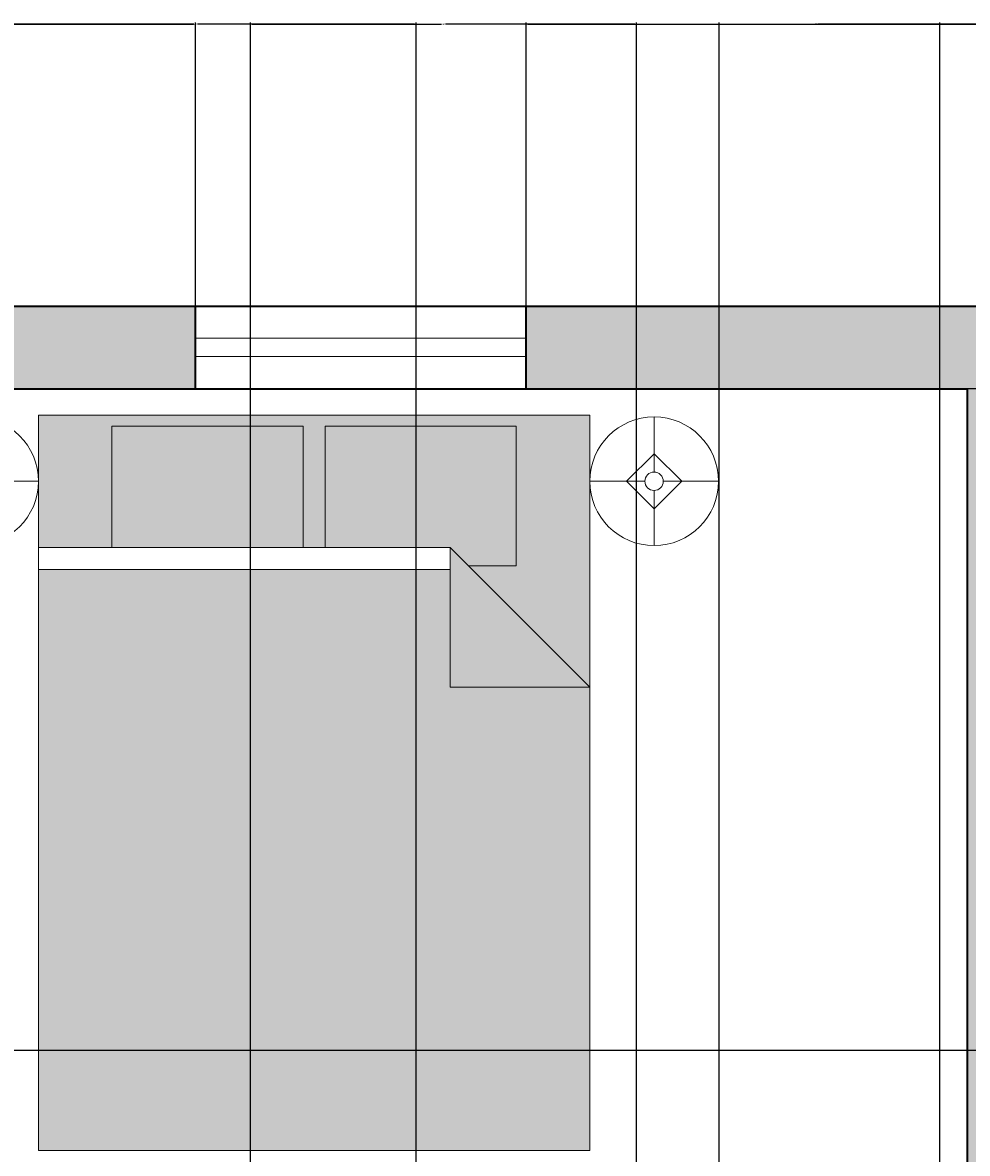
# Model space of a CAD drawing. Units: inches. Extents: x 1567 to 1964, y 1813 to 2447.
# Tile 15 of 28: x 1636 to 1738, y 2324 to 2447. Entities that reach past the tile are written whole.
import ezdxf

# ---------------------------------------------------------------- set-up
doc = ezdxf.new("R2010")
doc.units = ezdxf.units.IN
for name, color, linetype, lineweight in [('A-ANNO-DIMS', 2, 'Continuous', 18), ('A-FURN', 8, 'Continuous', 18), ('A-GLAZ', 4, 'Continuous', 18), ('A-WALL', 7, 'Continuous', 35)]:
    doc.layers.add(name, color=color, linetype=linetype, lineweight=lineweight)
doc.layers.add('A-FURN-PATT', color=252, linetype='Continuous', lineweight=13, true_color=0x939598)
doc.layers.add('A-WALL-PATT', color=251, linetype='Continuous', lineweight=13, true_color=0x636466)
doc.styles.get("Standard").update_dxf_attribs({"font": 'arial.ttf'})
doc.dimstyles.get("Standard").update_dxf_attribs({"dimtxt": 0.18, "dimasz": 0.18, "dimexe": 0.18, "dimexo": 0.0625, "dimgap": 0.09, "dimtad": 0, "dimtih": 1, "dimtoh": 1, "dimdec": 4, "dimzin": 0, "dimdsep": 46, "dimtxsty": 'Standard', "dimcen": 0.09, "dimadec": 0, "dimazin": 0, "dimtfac": 1, "dimtdec": 4, "dimtofl": 0, "dimtmove": 0, "dimatfit": 3, "dimfxl": 1, "dimtolj": 1, "dimtzin": 0, "dimarcsym": 0})

# ---------------------------------------------------------------- blocks, each defined once
blk = doc.blocks.new('Lamp - Table')
for p, q in [((0, 7), (0, 1)), ((0, 3), (-3, 0)), ((3, 0), (0, 3)), ((-1, 0), (-7, 0)), ((-3, 0), (0, -3)), ((0, -3), (3, 0)), ((1, 0), (7, 0)), ((0, -1), (0, -7))]:
    blk.add_line(p, q)
for radius in [7, 1]:
    blk.add_circle((0, 0), radius)
blk = doc.blocks.new('Bed - Queen')
for p, q in [((0, -80.00003), (0, 0)), ((0, 0), (59.99999, 0)), ((59.99999, 0), (59.99999, -80.00003)), ((7.99999, -1.2), (28.79998, -1.2)), ((7.99999, -14.4), (7.99999, -1.2)), ((28.79998, -1.2), (28.79998, -14.4)), ((31.19999, -1.2), (51.99999, -1.2)), ((31.19999, -14.4), (31.19999, -1.2)), ((51.99999, -1.2), (51.99999, -16.4)), ((0, -14.4), (44.8, -14.4)), ((59.99999, -29.6), (44.8, -14.4)), ((44.8, -14.4), (44.8, -29.6)), ((44.8, -16.8), (0, -16.8)), ((51.99999, -16.4), (46.79936, -16.4)), ((44.8, -29.6), (59.99999, -29.6)), ((59.99999, -80.00003), (0, -80.00003))]:
    blk.add_line(p, q)
blk = doc.blocks.new('WINDOW-36IN')
for p, q in [((0, 2), (36, 2)), ((0, 0), (36, 0))]:
    blk.add_line(p, q)
blk = doc.blocks.new('*D43')
at = {"layer": 'A-ANNO-DIMS', "color": 0, "lineweight": -2, "transparency": 16777216}
for p, q in [((1597.43, 2416.35), (1597.43, 2447.12)), ((1597.61, 2446.94), (1625.71, 2446.94)), ((1654.25, 2446.94), (1626.15, 2446.94)), ((1654.43, 2416.35), (1654.43, 2447.12))]:
    blk.add_line(p, q, dxfattribs=at)
at = {"layer": 'A-ANNO-DIMS', "color": 0, "transparency": 16777216}
for points in [[(1597.61, 2446.97), (1597.61, 2446.91), (1597.43, 2446.94)], [(1654.25, 2446.97), (1654.25, 2446.91), (1654.43, 2446.94)]]:
    blk.add_solid(points, dxfattribs=at)
at = {"layer": 'Defpoints', "color": 0, "transparency": 16777216}
for p in [(1654.43, 2446.94), (1597.43, 2416.29), (1654.43, 2416.29)]:
    blk.add_point(p, dxfattribs=at)
at = {"layer": 'A-ANNO-DIMS', "color": 0, "transparency": 16777216, "insert": (1625.93, 2446.94), "char_height": 0.18, "attachment_point": 5}
blk.add_mtext('\\A1;57', dxfattribs=at)
blk = doc.blocks.new('*D44')
at = {"layer": 'A-ANNO-DIMS', "color": 0, "lineweight": -2, "transparency": 16777216}
for p, q in [((1690.43, 2416.35), (1690.43, 2447.12)), ((1690.61, 2446.94), (1721.71, 2446.94)), ((1753.25, 2446.94), (1722.15, 2446.94)), ((1753.43, 2416.35), (1753.43, 2447.12))]:
    blk.add_line(p, q, dxfattribs=at)
at = {"layer": 'A-ANNO-DIMS', "color": 0, "transparency": 16777216}
for points in [[(1690.61, 2446.97), (1690.61, 2446.91), (1690.43, 2446.94)], [(1753.25, 2446.97), (1753.25, 2446.91), (1753.43, 2446.94)]]:
    blk.add_solid(points, dxfattribs=at)
at = {"layer": 'Defpoints', "color": 0, "transparency": 16777216}
for p in [(1753.43, 2446.94), (1690.43, 2416.29), (1753.43, 2416.29)]:
    blk.add_point(p, dxfattribs=at)
at = {"layer": 'A-ANNO-DIMS', "color": 0, "transparency": 16777216, "insert": (1721.93, 2446.94), "char_height": 0.18, "attachment_point": 5}
blk.add_mtext('\\A1;63', dxfattribs=at)
blk = doc.blocks.new('*D48')
at = {"layer": 'A-ANNO-DIMS', "color": 0, "lineweight": -2, "transparency": 16777216}
for p, q in [((1742.37, 2407.29), (1566.6, 2407.29)), ((1566.78, 2407.11), (1566.78, 2371.47)), ((1566.78, 2335.47), (1566.78, 2371.11)), ((1742.37, 2335.29), (1566.6, 2335.29))]:
    blk.add_line(p, q, dxfattribs=at)
at = {"layer": 'A-ANNO-DIMS', "color": 0, "transparency": 16777216}
for points in [[(1566.75, 2407.11), (1566.81, 2407.11), (1566.78, 2407.29)], [(1566.75, 2335.47), (1566.81, 2335.47), (1566.78, 2335.29)]]:
    blk.add_solid(points, dxfattribs=at)
at = {"layer": 'Defpoints', "color": 0, "transparency": 16777216}
for p in [(1742.43, 2407.29), (1566.78, 2335.29), (1742.43, 2335.29)]:
    blk.add_point(p, dxfattribs=at)
at = {"layer": 'A-ANNO-DIMS', "color": 0, "transparency": 16777216, "insert": (1566.78, 2371.29), "char_height": 0.18, "attachment_point": 5}
blk.add_mtext('\\A1;72', dxfattribs=at)
blk = doc.blocks.new('*D54')
at = {"layer": 'A-ANNO-DIMS', "color": 0, "lineweight": -2, "transparency": 16777216}
for p, q in [((1711.43, 1964.35), (1711.43, 2447.12)), ((1711.61, 2446.94), (1753.21, 2446.94)), ((1795.25, 2446.94), (1753.65, 2446.94)), ((1795.43, 1964.35), (1795.43, 2447.12))]:
    blk.add_line(p, q, dxfattribs=at)
at = {"layer": 'A-ANNO-DIMS', "color": 0, "transparency": 16777216}
for points in [[(1711.61, 2446.97), (1711.61, 2446.91), (1711.43, 2446.94)], [(1795.25, 2446.97), (1795.25, 2446.91), (1795.43, 2446.94)]]:
    blk.add_solid(points, dxfattribs=at)
at = {"layer": 'Defpoints', "color": 0, "transparency": 16777216}
for p in [(1795.43, 2446.94), (1711.43, 1964.29), (1795.43, 1964.29)]:
    blk.add_point(p, dxfattribs=at)
at = {"layer": 'A-ANNO-DIMS', "color": 0, "transparency": 16777216, "insert": (1753.43, 2446.94), "char_height": 0.18, "attachment_point": 5}
blk.add_mtext('\\A1;84', dxfattribs=at)
blk = doc.blocks.new('*D57')
at = {"layer": 'A-ANNO-DIMS', "color": 0, "lineweight": -2, "transparency": 16777216}
for p, q in [((1630.43, 2127.35), (1630.43, 2447.12)), ((1630.61, 2446.94), (1654.21, 2446.94)), ((1678.25, 2446.94), (1654.65, 2446.94)), ((1678.43, 2127.35), (1678.43, 2447.12))]:
    blk.add_line(p, q, dxfattribs=at)
at = {"layer": 'A-ANNO-DIMS', "color": 0, "transparency": 16777216}
for points in [[(1630.61, 2446.97), (1630.61, 2446.91), (1630.43, 2446.94)], [(1678.25, 2446.97), (1678.25, 2446.91), (1678.43, 2446.94)]]:
    blk.add_solid(points, dxfattribs=at)
at = {"layer": 'Defpoints', "color": 0, "transparency": 16777216}
for p in [(1678.43, 2446.94), (1630.43, 2127.29), (1678.43, 2127.29)]:
    blk.add_point(p, dxfattribs=at)
at = {"layer": 'A-ANNO-DIMS', "color": 0, "transparency": 16777216, "insert": (1654.43, 2446.94), "char_height": 0.18, "attachment_point": 5}
blk.add_mtext('\\A1;48', dxfattribs=at)
blk = doc.blocks.new('*D60')
at = {"layer": 'A-ANNO-DIMS', "color": 0, "lineweight": -2, "transparency": 16777216}
for p, q in [((1660.43, 2063.35), (1660.43, 2447.12)), ((1660.61, 2446.94), (1681.21, 2446.94)), ((1702.25, 2446.94), (1681.65, 2446.94)), ((1702.43, 2063.35), (1702.43, 2447.12))]:
    blk.add_line(p, q, dxfattribs=at)
at = {"layer": 'A-ANNO-DIMS', "color": 0, "transparency": 16777216}
for points in [[(1660.61, 2446.97), (1660.61, 2446.91), (1660.43, 2446.94)], [(1702.25, 2446.97), (1702.25, 2446.91), (1702.43, 2446.94)]]:
    blk.add_solid(points, dxfattribs=at)
at = {"layer": 'Defpoints', "color": 0, "transparency": 16777216}
for p in [(1660.43, 2446.94), (1660.43, 2063.29), (1702.43, 2063.29)]:
    blk.add_point(p, dxfattribs=at)
at = {"layer": 'A-ANNO-DIMS', "color": 0, "transparency": 16777216, "insert": (1681.43, 2446.94), "char_height": 0.18, "attachment_point": 5}
blk.add_mtext('\\A1;42', dxfattribs=at)
blk = doc.blocks.new('*D63')
at = {"layer": 'A-ANNO-DIMS', "color": 0, "lineweight": -2, "transparency": 16777216}
for p, q in [((1735.43, 1988.35), (1735.43, 2447.12)), ((1735.61, 2446.94), (1753.21, 2446.94)), ((1771.25, 2446.94), (1753.65, 2446.94)), ((1771.43, 1988.35), (1771.43, 2447.12))]:
    blk.add_line(p, q, dxfattribs=at)
at = {"layer": 'A-ANNO-DIMS', "color": 0, "transparency": 16777216}
for points in [[(1735.61, 2446.97), (1735.61, 2446.91), (1735.43, 2446.94)], [(1771.25, 2446.97), (1771.25, 2446.91), (1771.43, 2446.94)]]:
    blk.add_solid(points, dxfattribs=at)
at = {"layer": 'Defpoints', "color": 0, "transparency": 16777216}
for p in [(1771.43, 2446.94), (1735.43, 1988.29), (1771.43, 1988.29)]:
    blk.add_point(p, dxfattribs=at)
at = {"layer": 'A-ANNO-DIMS', "color": 0, "transparency": 16777216, "insert": (1753.43, 2446.94), "char_height": 0.18, "attachment_point": 5}
blk.add_mtext('\\A1;36', dxfattribs=at)
blk = doc.blocks.new('*D64')
at = {"layer": 'A-ANNO-DIMS', "color": 0, "lineweight": -2, "transparency": 16777216}
for p, q in [((1711.43, 2055.85), (1711.43, 2447.12)), ((1711.61, 2446.94), (1723.21, 2446.94)), ((1735.25, 2446.94), (1723.65, 2446.94)), ((1735.43, 2055.85), (1735.43, 2447.12))]:
    blk.add_line(p, q, dxfattribs=at)
at = {"layer": 'A-ANNO-DIMS', "color": 0, "transparency": 16777216}
for points in [[(1711.61, 2446.97), (1711.61, 2446.91), (1711.43, 2446.94)], [(1735.25, 2446.97), (1735.25, 2446.91), (1735.43, 2446.94)]]:
    blk.add_solid(points, dxfattribs=at)
at = {"layer": 'Defpoints', "color": 0, "transparency": 16777216}
for p in [(1735.43, 2446.94), (1711.43, 2055.79), (1735.43, 2055.79)]:
    blk.add_point(p, dxfattribs=at)
at = {"layer": 'A-ANNO-DIMS', "color": 0, "transparency": 16777216, "insert": (1723.43, 2446.94), "char_height": 0.18, "attachment_point": 5}
blk.add_mtext('\\A1;24', dxfattribs=at)

msp = doc.modelspace()

# ---------------------------------------------------------------- hatches: boundary and pattern name
at = {"layer": 'A-FURN-PATT'}
h = msp.add_hatch(color=256, dxfattribs=at)
h.dxf.hatch_style = 1
h.paths.add_polyline_path([(1621.2532, 2242.0229), (1643.7811, 2241.7239), (1643.8607, 2247.7234), (1617.863, 2248.0685, 0.19047621), (1616.7481, 2164.0759), (1642.7458, 2163.7308), (1642.8254, 2169.7302), (1620.2975, 2170.0293, -0.15194781)])
h.paths.add_polyline_path([(1673.5306, 2249.6607), (1653.8509, 2249.6607), (1653.8509, 2248.5031, 0.11764706), (1673.5306, 2248.5031)])
h.paths.add_polyline_path([(1706.0889, 2249.6607), (1686.4092, 2249.6607), (1686.4092, 2248.5031, 0.11764706), (1706.0889, 2248.5031)])
h.paths.add_polyline_path([(1782.4511, 2227.4197), (1766.4511, 2227.4197), (1766.2949, 2226.4197), (1782.6074, 2226.4197)])
h.paths.add_polyline_path([(1810.4511, 2227.4197), (1794.4511, 2227.4197), (1794.2949, 2226.4197), (1810.6074, 2226.4197)])
h.paths.add_polyline_path([(1743.9511, 2208.076), (1742.9511, 2207.9197), (1742.9511, 2191.9197), (1743.9511, 2191.7635)])
h.paths.add_polyline_path([(1782.6074, 2173.4197), (1766.2949, 2173.4197), (1766.4511, 2172.4197), (1782.4511, 2172.4197)])
h.paths.add_polyline_path([(1810.6074, 2173.4197), (1794.2949, 2173.4197), (1794.4511, 2172.4197), (1810.4511, 2172.4197)])
h.paths.add_polyline_path([(1861.053, 2006.5071), (1845.8531, 2006.5071), (1861.053, 1991.3071)])
h.paths.add_polyline_path([(1905.853, 1993.7071), (1861.053, 1993.7071), (1861.053, 1991.3071), (1905.853, 1991.3071)])
h.paths.add_polyline_path([(1919.7245, 2257.29, 0.50000012), (1918.7245, 2258.29), (1901.7245, 2258.29, 0.50000012), (1900.7245, 2257.29), (1900.7245, 2253.29, 0.50000012), (1901.7245, 2252.29), (1918.7245, 2252.29, 0.50000012), (1919.7245, 2253.29)])
h.paths.add_polyline_path([(1875.9094, 2391.0204), (1875.9094, 2375.8204), (1891.1093, 2375.8204)], flags=17)
h.paths.add_polyline_path([(1891.1093, 2405.4204), (1831.1094, 2405.4204), (1831.1094, 2391.0204), (1839.1093, 2391.0204), (1839.1093, 2404.2204), (1859.9093, 2404.2204), (1859.9093, 2391.0204), (1862.3093, 2391.0204), (1862.3093, 2404.2204), (1883.1093, 2404.2204), (1883.1093, 2389.0204), (1877.9094, 2389.0204), (1891.1093, 2375.8204)])
h.paths.add_polyline_path([(1682.1402, 2390.0316), (1682.1402, 2374.8316), (1697.3402, 2374.8316)], flags=17)
h.paths.add_polyline_path([(1697.3402, 2404.4316), (1637.3402, 2404.4316), (1637.3402, 2390.0316), (1645.3402, 2390.0316), (1645.3402, 2403.2316), (1666.1402, 2403.2316), (1666.1402, 2390.0316), (1668.5402, 2390.0316), (1668.5402, 2403.2316), (1689.3402, 2403.2316), (1689.3402, 2388.0316), (1684.1402, 2388.0316), (1697.3402, 2374.8316)])
h = msp.add_hatch(color=256, dxfattribs=at)
h.dxf.hatch_style = 1
h.paths.add_polyline_path([(1666.1402, 2403.2316), (1645.3402, 2403.2316), (1645.3402, 2390.0316), (1666.1402, 2390.0316)])
h.paths.add_polyline_path([(1689.3402, 2403.2316), (1668.5402, 2403.2316), (1668.5402, 2390.0316), (1682.1402, 2390.0316), (1684.1402, 2388.0316), (1689.3402, 2388.0316)])
h.paths.add_polyline_path([(1859.9093, 2404.2204), (1839.1093, 2404.2204), (1839.1093, 2391.0204), (1859.9093, 2391.0204)])
h.paths.add_polyline_path([(1883.1093, 2404.2204), (1862.3093, 2404.2204), (1862.3093, 2391.0204), (1875.9094, 2391.0204), (1877.9094, 2389.0204), (1883.1093, 2389.0204)])
h = msp.add_hatch(color=256, dxfattribs=at)
h.dxf.hatch_style = 1
h.paths.add_polyline_path([(1697.3402, 2374.8316), (1682.1402, 2374.8316), (1682.1402, 2387.6316), (1637.3402, 2387.6316), (1637.3402, 2324.4315), (1697.3402, 2324.4315)])
h.paths.add_polyline_path([(1891.1093, 2375.8204), (1875.9094, 2375.8204), (1875.9094, 2388.6204), (1831.1094, 2388.6204), (1831.1094, 2325.4204), (1891.1093, 2325.4204)])
h.paths.add_polyline_path([(1702.5611, 2206.8057), (1702.5611, 2210.8057), (1699.7395, 2209.9436), (1697.013, 2209.2403), (1694.3857, 2208.6763), (1691.8615, 2208.2326), (1689.4443, 2207.8896), (1687.1381, 2207.6282), (1684.9469, 2207.4289), (1682.8747, 2207.2725), (1680.9233, 2207.1425), (1679.0865, 2207.0339), (1677.3558, 2206.9445), (1675.7229, 2206.8719), (1674.1794, 2206.8141), (1672.7169, 2206.7688), (1671.327, 2206.7339), (1670.0014, 2206.707), (1668.7314, 2206.6866), (1667.5072, 2206.6732), (1666.3188, 2206.668), (1665.1561, 2206.6722), (1664.009, 2206.6869), (1662.8675, 2206.7133), (1661.7215, 2206.7525), (1660.5611, 2206.8057), (1660.5611, 2202.8057), (1661.9932, 2202.9556), (1663.3314, 2203.0744), (1664.5899, 2203.1671), (1665.7831, 2203.2385), (1666.9254, 2203.2935), (1668.0311, 2203.3368), (1669.1145, 2203.3734), (1670.1902, 2203.4081), (1671.2724, 2203.4451), (1672.3759, 2203.4866), (1673.5155, 2203.534), (1674.706, 2203.5887), (1675.9621, 2203.6523), (1677.2986, 2203.7262), (1678.7304, 2203.8118), (1680.2722, 2203.9108), (1681.947, 2204.0272), (1683.8108, 2204.1769), (1685.9279, 2204.3782), (1688.3626, 2204.6496), (1691.179, 2205.0096), (1694.4413, 2205.4767), (1698.214, 2206.0692)])
h.paths.add_polyline_path([(1702.5611, 2218.8057), (1701.9821, 2217.9383), (1701.3316, 2217.191), (1700.6091, 2216.5515), (1699.8141, 2216.0071), (1698.946, 2215.5454), (1698.0041, 2215.1536), (1696.9879, 2214.8194), (1695.8969, 2214.5301), (1694.7328, 2214.2753), (1693.5072, 2214.0522), (1692.2339, 2213.8602), (1690.9266, 2213.6989), (1689.5994, 2213.5675), (1688.266, 2213.4654), (1686.9402, 2213.392), (1685.636, 2213.3467), (1684.3619, 2213.3287), (1683.1053, 2213.3361), (1681.8482, 2213.3668), (1680.5727, 2213.4187), (1679.2608, 2213.4898), (1677.8948, 2213.5779), (1676.4565, 2213.6811), (1674.9282, 2213.7971), (1673.2982, 2213.9236), (1671.5804, 2214.0573), (1669.795, 2214.1945), (1667.9622, 2214.3316), (1666.1022, 2214.4649), (1664.2352, 2214.5908), (1662.3814, 2214.7056), (1660.5611, 2214.8057), (1660.5611, 2206.8057), (1661.7215, 2206.7525), (1662.8675, 2206.7133), (1664.009, 2206.6869), (1665.1561, 2206.6722), (1666.3188, 2206.668), (1667.5072, 2206.6732), (1668.7314, 2206.6866), (1670.0014, 2206.707), (1671.327, 2206.7339), (1672.7169, 2206.7688), (1674.1794, 2206.8141), (1675.7229, 2206.8719), (1677.3558, 2206.9445), (1679.0865, 2207.0339), (1680.9233, 2207.1425), (1682.8747, 2207.2725), (1684.9469, 2207.4289), (1687.1381, 2207.6282), (1689.4443, 2207.8896), (1691.8615, 2208.2326), (1694.3857, 2208.6763), (1697.013, 2209.2403), (1699.7395, 2209.9436), (1702.5611, 2210.8057)])
h.paths.add_polyline_path([(1700.6091, 2216.5515), (1701.3316, 2217.191), (1701.9821, 2217.9383), (1702.5611, 2218.8057), (1702.5611, 2222.8057), (1689.452, 2222.8057), (1689.0171, 2222.4556), (1688.4521, 2222.0354), (1687.7806, 2221.5662), (1687.0235, 2221.067), (1686.2019, 2220.5566), (1685.3367, 2220.0541), (1684.4491, 2219.5785), (1683.56, 2219.1486), (1682.6867, 2218.7795), (1681.8312, 2218.4692), (1680.9918, 2218.212), (1680.1667, 2218.0019), (1679.3541, 2217.833), (1678.5524, 2217.6995), (1677.7597, 2217.5954), (1676.9744, 2217.5149), (1676.1942, 2217.4531), (1675.4146, 2217.4093), (1674.6309, 2217.384), (1673.8381, 2217.3774), (1673.0313, 2217.39), (1672.2056, 2217.4221), (1671.3562, 2217.4741), (1670.4782, 2217.5463), (1669.5642, 2217.639), (1668.5968, 2217.7516), (1667.5562, 2217.8833), (1666.4226, 2218.0336), (1665.1761, 2218.2017), (1663.7969, 2218.3869), (1662.2651, 2218.5885), (1660.5611, 2218.8057), (1660.5611, 2214.8057), (1662.3814, 2214.7056), (1664.2352, 2214.5908), (1666.1022, 2214.4649), (1667.9622, 2214.3316), (1669.795, 2214.1945), (1671.5804, 2214.0573), (1673.2982, 2213.9236), (1674.9282, 2213.7971), (1676.4565, 2213.6811), (1677.8948, 2213.5779), (1679.2608, 2213.4898), (1680.5727, 2213.4187), (1681.8482, 2213.3668), (1683.1053, 2213.3361), (1684.3619, 2213.3287), (1685.636, 2213.3467), (1686.9402, 2213.392), (1688.266, 2213.4654), (1689.5994, 2213.5675), (1690.9266, 2213.6989), (1692.2339, 2213.8602), (1693.5072, 2214.0522), (1694.7328, 2214.2753), (1695.8969, 2214.5301), (1696.9879, 2214.8194), (1698.0041, 2215.1536), (1698.946, 2215.5454), (1699.8141, 2216.0071)])
h.paths.add_polyline_path([(1687.0235, 2221.067), (1687.7806, 2221.5662), (1688.4521, 2222.0354), (1689.0171, 2222.4556), (1689.452, 2222.8057), (1660.5611, 2222.8057), (1660.5611, 2218.8057), (1662.2651, 2218.5885), (1663.7969, 2218.3869), (1665.1761, 2218.2017), (1666.4226, 2218.0336), (1667.5562, 2217.8833), (1668.5968, 2217.7516), (1669.5642, 2217.639), (1670.4782, 2217.5463), (1671.3562, 2217.4741), (1672.2056, 2217.4221), (1673.0313, 2217.39), (1673.8381, 2217.3774), (1674.6309, 2217.384), (1675.4146, 2217.4093), (1676.1942, 2217.4531), (1676.9744, 2217.5149), (1677.7597, 2217.5954), (1678.5524, 2217.6995), (1679.3541, 2217.833), (1680.1667, 2218.0019), (1680.9918, 2218.212), (1681.8312, 2218.4692), (1682.6867, 2218.7795), (1683.56, 2219.1486), (1684.4491, 2219.5785), (1685.3367, 2220.0541), (1686.2019, 2220.5566)], flags=17)
h.paths.add_polyline_path([(1702.5611, 2198.8057), (1698.9289, 2199.2412), (1695.8472, 2199.5774), (1693.2166, 2199.8257), (1690.9377, 2199.9973), (1688.9111, 2200.1033), (1687.0375, 2200.155), (1685.2174, 2200.1637), (1683.3514, 2200.1406), (1681.3514, 2200.0941), (1679.1736, 2200.0225), (1676.7858, 2199.921), (1674.1554, 2199.7852), (1671.2502, 2199.6103), (1668.0377, 2199.3919), (1664.4854, 2199.1252), (1660.5611, 2198.8057), (1660.5611, 2194.8057), (1662.2697, 2194.9771), (1663.9673, 2195.0999), (1665.6339, 2195.1809), (1667.2495, 2195.227), (1668.7941, 2195.2449), (1670.2478, 2195.2414), (1671.5906, 2195.2233), (1672.8026, 2195.1974), (1673.8739, 2195.1689), (1674.8359, 2195.1364), (1675.7302, 2195.0967), (1676.5982, 2195.0469), (1677.4817, 2194.9838), (1678.422, 2194.9043), (1679.4609, 2194.8055), (1680.6397, 2194.6842), (1682.005, 2194.5341), (1683.6223, 2194.335), (1685.562, 2194.0637), (1687.8945, 2193.6967), (1690.6902, 2193.2108), (1694.0196, 2192.5826), (1697.9531, 2191.7887), (1702.5611, 2190.8057)])
h.paths.add_polyline_path([(1702.5611, 2206.8057), (1698.214, 2206.0692), (1694.4413, 2205.4767), (1691.179, 2205.0096), (1688.3626, 2204.6496), (1685.9279, 2204.3782), (1683.8108, 2204.1769), (1681.947, 2204.0272), (1680.2722, 2203.9108), (1678.7304, 2203.8118), (1677.2986, 2203.7262), (1675.9621, 2203.6523), (1674.706, 2203.5887), (1673.5155, 2203.534), (1672.3759, 2203.4866), (1671.2724, 2203.4451), (1670.1902, 2203.4081), (1669.1145, 2203.3734), (1668.0311, 2203.3368), (1666.9254, 2203.2935), (1665.7831, 2203.2385), (1664.5899, 2203.1671), (1663.3314, 2203.0744), (1661.9932, 2202.9556), (1660.5611, 2202.8057), (1660.5611, 2198.8057), (1664.4854, 2199.1252), (1668.0377, 2199.3919), (1671.2502, 2199.6103), (1674.1554, 2199.7852), (1676.7858, 2199.921), (1679.1736, 2200.0225), (1681.3514, 2200.0941), (1683.3514, 2200.1406), (1685.2174, 2200.1637), (1687.0375, 2200.155), (1688.9111, 2200.1033), (1690.9377, 2199.9973), (1693.2166, 2199.8257), (1695.8472, 2199.5774), (1698.9289, 2199.2412), (1702.5611, 2198.8057)])
h.paths.add_polyline_path([(1702.5611, 2190.8057), (1697.9531, 2191.7887), (1694.0196, 2192.5826), (1690.6902, 2193.2108), (1687.8945, 2193.6967), (1685.562, 2194.0637), (1683.6223, 2194.335), (1682.005, 2194.5341), (1680.6397, 2194.6842), (1679.4609, 2194.8055), (1678.422, 2194.9043), (1677.4817, 2194.9838), (1676.5982, 2195.0469), (1675.7302, 2195.0967), (1674.8359, 2195.1364), (1673.8739, 2195.1689), (1672.8026, 2195.1974), (1671.5906, 2195.2233), (1670.2478, 2195.2414), (1668.7941, 2195.2449), (1667.2495, 2195.227), (1665.6339, 2195.1809), (1663.9673, 2195.0999), (1662.2697, 2194.9771), (1660.5611, 2194.8057), (1660.5611, 2190.8057), (1665.9637, 2190.2699), (1670.5105, 2189.7867), (1674.3035, 2189.3504), (1677.4445, 2188.9552), (1680.0354, 2188.5951), (1682.1782, 2188.2644), (1683.9747, 2187.9571), (1685.5268, 2187.6675), (1686.9225, 2187.3901), (1688.1943, 2187.1216), (1689.3606, 2186.859), (1690.4399, 2186.5993), (1691.4508, 2186.3396), (1692.4118, 2186.0769), (1693.3413, 2185.8084), (1694.2579, 2185.531), (1695.1786, 2185.2422), (1696.1142, 2184.9406), (1697.0739, 2184.6252), (1698.0671, 2184.2949), (1699.1032, 2183.9489), (1700.1913, 2183.586), (1701.3408, 2183.2053), (1702.5611, 2182.8057)])
h.paths.add_polyline_path([(1702.5611, 2182.8057), (1701.3408, 2183.2053), (1700.1913, 2183.586), (1699.1032, 2183.9489), (1698.0671, 2184.2949), (1697.0739, 2184.6252), (1696.1142, 2184.9406), (1695.1786, 2185.2422), (1694.2579, 2185.531), (1693.3413, 2185.8084), (1692.4118, 2186.0769), (1691.4508, 2186.3396), (1690.4399, 2186.5993), (1689.3606, 2186.859), (1688.1943, 2187.1216), (1686.9225, 2187.3901), (1685.5268, 2187.6675), (1683.9747, 2187.9571), (1682.1782, 2188.2644), (1680.0354, 2188.5951), (1677.4445, 2188.9552), (1674.3035, 2189.3504), (1670.5105, 2189.7867), (1665.9637, 2190.2699), (1660.5611, 2190.8057), (1660.5611, 2186.8057), (1663.5709, 2186.52), (1666.0965, 2186.2414), (1668.1979, 2185.9698), (1669.9351, 2185.7048), (1671.3681, 2185.446), (1672.5568, 2185.1931), (1673.5613, 2184.9458), (1674.4415, 2184.7037), (1675.2485, 2184.4664), (1675.9976, 2184.2328), (1677.0295, 2183.8907), (1678.2492, 2183.4332), (1679.354, 2182.9669), (1680.4123, 2182.4724), (1681.3757, 2181.9718), (1682.2435, 2181.4594), (1683.1864, 2180.8057), (1702.5611, 2180.8057)])
h.paths.add_polyline_path([(1677.3469, 2183.7716), (1676.6949, 2184.0016), (1675.9976, 2184.2328), (1675.2485, 2184.4664), (1674.4415, 2184.7037), (1673.5613, 2184.9458), (1672.5568, 2185.1931), (1671.3681, 2185.446), (1669.9351, 2185.7048), (1668.1979, 2185.9698), (1666.0965, 2186.2414), (1663.5709, 2186.52), (1660.5611, 2186.8057), (1660.5611, 2180.8057), (1683.1506, 2180.8057), (1682.802, 2181.0722), (1682.4264, 2181.3326), (1682.0201, 2181.5913), (1681.586, 2181.8476), (1681.1268, 2182.1011), (1680.6453, 2182.3513), (1680.1443, 2182.5976), (1679.6266, 2182.8395), (1679.0933, 2183.0769), (1678.5398, 2183.3105), (1677.9598, 2183.5417)], flags=17)
h.paths.add_polyline_path([(1824.4511, 2199.9016), (1824.089, 2199.9302), (1824.0595, 2199.9372), (1824.0397, 2199.9406), (1823.5413, 2200.0576), (1823.4095, 2200.0864), (1823.0664, 2200.1559), (1822.6419, 2200.2361), (1822.1519, 2200.3222), (1821.6126, 2200.4093), (1821.0401, 2200.4925), (1820.4505, 2200.5669), (1819.8599, 2200.6276), (1819.2845, 2200.6697), (1818.7366, 2200.6896), (1818.2141, 2200.688), (1817.7112, 2200.6668), (1817.222, 2200.6281), (1816.7405, 2200.5737), (1816.261, 2200.5057), (1815.7776, 2200.4259), (1815.2845, 2200.3364), (1814.3007, 2200.149), (1813.3315, 2199.9765), (1812.406, 2199.8514), (1811.6868, 2199.7739), (1810.8992, 2199.7121), (1810.0345, 2199.6697), (1809.0854, 2199.6497), (1808.0514, 2199.6502), (1806.9334, 2199.6683), (1805.7324, 2199.701), (1804.4493, 2199.7454), (1803.0852, 2199.7986), (1801.641, 2199.8577), (1800.1178, 2199.9197), (1798.5134, 2199.9818), (1796.8144, 2200.0415), (1795.004, 2200.0962), (1793.0657, 2200.1437), (1790.9828, 2200.1814), (1788.7389, 2200.2068), (1786.3171, 2200.2177), (1783.7011, 2200.2114), (1780.8715, 2200.185), (1777.7988, 2200.1326), (1774.4506, 2200.0481), (1770.7948, 2199.9249), (1766.7992, 2199.7569), (1762.4316, 2199.5376), (1757.6596, 2199.2606), (1752.4511, 2198.9197), (1752.4511, 2193.4197), (1761.2668, 2193.6071), (1768.3671, 2193.7934), (1773.9821, 2193.9778), (1778.3417, 2194.1593), (1781.6759, 2194.3369), (1784.2148, 2194.5096), (1786.1882, 2194.6764), (1787.8261, 2194.8364), (1789.3219, 2194.9887), (1790.7226, 2195.1333), (1792.0383, 2195.27), (1793.2792, 2195.3989), (1794.4557, 2195.52), (1795.5781, 2195.6333), (1796.6564, 2195.7387), (1797.7011, 2195.8364), (1798.7216, 2195.9259), (1799.7245, 2196.0057), (1800.7158, 2196.0737), (1801.7011, 2196.1281), (1802.6865, 2196.1668), (1803.6777, 2196.188), (1804.6806, 2196.1896), (1805.7011, 2196.1697), (1806.7423, 2196.1273), (1807.7962, 2196.0643), (1808.852, 2195.9837), (1809.899, 2195.8885), (1810.9265, 2195.7815), (1811.9238, 2195.6658), (1812.88, 2195.5442), (1813.7845, 2195.4197), (1814.6296, 2195.2948), (1815.4205, 2195.1704), (1816.1656, 2195.0469), (1816.873, 2194.9249), (1817.5511, 2194.8049), (1818.2083, 2194.6873), (1818.8527, 2194.5726), (1819.4928, 2194.4614), (1820.1348, 2194.3554), (1820.7773, 2194.2615), (1821.4169, 2194.1882), (1822.0501, 2194.1437), (1822.6735, 2194.1363), (1823.2838, 2194.1743), (1823.8775, 2194.266), (1824.4511, 2194.4197)])
h.paths.add_polyline_path([(1821.4716, 2190.5098), (1820.4303, 2190.5708), (1819.3811, 2190.6415), (1818.3339, 2190.7186), (1817.2985, 2190.7986), (1816.2845, 2190.8781), (1815.2976, 2190.9542), (1814.3274, 2191.0259), (1813.3592, 2191.0927), (1812.3782, 2191.1541), (1811.3699, 2191.2097), (1810.3196, 2191.2589), (1809.2127, 2191.3013), (1808.0345, 2191.3364), (1806.7708, 2191.3634), (1805.4094, 2191.3807), (1803.9387, 2191.3862), (1802.3469, 2191.3781), (1800.6223, 2191.3543), (1798.7532, 2191.313), (1796.7278, 2191.2521), (1794.5344, 2191.1697), (1792.128, 2191.0648), (1789.33, 2190.9393), (1785.9285, 2190.7962), (1781.7115, 2190.6385), (1776.4672, 2190.469), (1769.9836, 2190.2908), (1762.0489, 2190.1067), (1752.4511, 2189.9197), (1752.4511, 2185.4197), (1758.363, 2185.5846), (1763.4179, 2185.7075), (1767.7199, 2185.7933), (1771.373, 2185.8468), (1774.4811, 2185.873), (1777.1484, 2185.8768), (1779.4787, 2185.8629), (1781.5761, 2185.8364), (1783.5287, 2185.8014), (1785.3606, 2185.7596), (1787.0802, 2185.7119), (1788.6959, 2185.6593), (1790.2158, 2185.6028), (1791.6484, 2185.5434), (1793.0018, 2185.4821), (1794.2844, 2185.4197), (1795.5065, 2185.3576), (1796.6861, 2185.298), (1797.8433, 2185.2432), (1798.998, 2185.1958), (1800.1703, 2185.1581), (1801.3801, 2185.1326), (1802.6476, 2185.1218), (1803.9928, 2185.1281), (1805.4444, 2185.1555), (1807.0663, 2185.2147), (1808.9315, 2185.3178), (1811.1126, 2185.477), (1813.6823, 2185.7046), (1816.7135, 2186.0128), (1820.2788, 2186.4138), (1824.4511, 2186.9197), (1824.4511, 2190.4197), (1823.4918, 2190.4309), (1822.4954, 2190.4621)])
h.paths.add_polyline_path([(1797.3762, 2216.0584), (1797.6199, 2216.2267), (1797.9558, 2216.3355), (1798.3017, 2216.3703), (1798.5761, 2216.3781), (1798.8974, 2216.3703), (1799.2714, 2216.3468), (1799.704, 2216.3078), (1800.2011, 2216.2531), (1800.7695, 2216.1829), (1801.4205, 2216.0981), (1802.1662, 2215.9996), (1803.0188, 2215.8885), (1803.9906, 2215.7656), (1805.0937, 2215.632), (1806.3404, 2215.4886), (1807.7428, 2215.3364), (1809.3101, 2215.1764), (1811.039, 2215.0096), (1812.9232, 2214.8369), (1814.9563, 2214.6593), (1817.132, 2214.4778), (1819.444, 2214.2934), (1821.8858, 2214.1071), (1824.4511, 2213.9197), (1824.4511, 2217.9197), (1752.4511, 2217.9197), (1752.4511, 2214.9197), (1757.2739, 2214.8973), (1761.6432, 2214.8338), (1765.5973, 2214.7352), (1769.1751, 2214.6072), (1772.4149, 2214.4559), (1775.3554, 2214.2869), (1778.0352, 2214.1063), (1780.4928, 2213.9197), (1782.7607, 2213.7329), (1784.8476, 2213.5499), (1786.7557, 2213.3748), (1788.4876, 2213.2114), (1790.0456, 2213.0636), (1791.4322, 2212.9354), (1792.6499, 2212.8305), (1793.7011, 2212.7531), (1794.5904, 2212.7059), (1795.3313, 2212.688), (1795.9394, 2212.6974), (1796.4303, 2212.7322), (1796.8196, 2212.7905), (1797.123, 2212.8703), (1797.356, 2212.9695), (1797.5344, 2213.0864), (1797.6716, 2213.2187), (1797.7727, 2213.3637), (1797.8406, 2213.5185), (1797.8782, 2213.6801), (1797.8884, 2213.8457), (1797.8743, 2214.0122), (1797.8386, 2214.1767), (1797.7844, 2214.3364), (1797.7149, 2214.4889), (1797.6347, 2214.6346), (1797.5486, 2214.7744), (1797.3327, 2215.109), (1797.178, 2215.4303), (1797.1896, 2215.7939)])
h.paths.add_polyline_path([(1804.7872, 2210.6789), (1804.546, 2211.022), (1804.3512, 2211.3917), (1804.2466, 2211.7546), (1804.2574, 2212.0998), (1804.4058, 2212.4178), (1804.7068, 2212.7007), (1805.1359, 2212.9124), (1805.5279, 2212.9926), (1805.8136, 2213.0154), (1806.1178, 2213.0031), (1806.4405, 2212.9529), (1806.7929, 2212.867), (1807.1893, 2212.7489), (1807.6438, 2212.602), (1808.1706, 2212.4297), (1808.7838, 2212.2355), (1809.4976, 2212.0227), (1810.3261, 2211.7947), (1811.2868, 2211.5533), (1812.4101, 2211.2928), (1813.7297, 2211.0059), (1815.2793, 2210.6854), (1817.0925, 2210.3238), (1819.2031, 2209.9139), (1821.6447, 2209.4483), (1824.4511, 2208.9197), (1824.4511, 2213.9197), (1821.8858, 2214.1071), (1819.444, 2214.2934), (1817.132, 2214.4778), (1814.9563, 2214.6593), (1812.9232, 2214.8369), (1811.039, 2215.0096), (1809.3101, 2215.1764), (1807.7428, 2215.3364), (1806.3404, 2215.4886), (1805.0937, 2215.632), (1803.9906, 2215.7656), (1803.0188, 2215.8885), (1802.1662, 2215.9996), (1801.4205, 2216.0981), (1800.7695, 2216.1829), (1800.2011, 2216.2531), (1799.704, 2216.3078), (1799.2714, 2216.3468), (1798.8974, 2216.3703), (1798.5761, 2216.3781), (1798.3017, 2216.3703), (1798.0683, 2216.3468), (1797.87, 2216.3078), (1797.7011, 2216.2531), (1797.5566, 2216.1831), (1797.4355, 2216.0994), (1797.3378, 2216.004), (1797.2636, 2215.8989), (1797.2128, 2215.7859), (1797.1855, 2215.6671), (1797.1816, 2215.5444), (1797.2011, 2215.4197), (1797.2433, 2215.2946), (1797.304, 2215.1684), (1797.3783, 2215.0403), (1797.4615, 2214.9093), (1797.6718, 2214.5836), (1797.8218, 2214.2545), (1797.8933, 2213.9247), (1797.8728, 2213.5918), (1797.7366, 2213.2814), (1797.4586, 2213.0132), (1797.123, 2212.8703), (1796.8196, 2212.7905), (1796.4303, 2212.7322), (1795.9394, 2212.6974), (1795.3313, 2212.688), (1794.5904, 2212.7059), (1793.7011, 2212.7531), (1792.6499, 2212.8305), (1791.4322, 2212.9354), (1790.0456, 2213.0636), (1788.4876, 2213.2114), (1786.7557, 2213.3748), (1784.8476, 2213.5499), (1782.7607, 2213.7329), (1780.4928, 2213.9197), (1778.0352, 2214.1063), (1775.3554, 2214.2869), (1772.4149, 2214.4559), (1769.1751, 2214.6072), (1765.5973, 2214.7352), (1761.6432, 2214.8338), (1757.2739, 2214.8973), (1752.4511, 2214.9197), (1752.4511, 2209.9197), (1759.4745, 2210.0625), (1765.2786, 2210.1242), (1770.027, 2210.1175), (1773.8834, 2210.0551), (1777.0112, 2209.9498), (1779.5741, 2209.8143), (1781.7357, 2209.6611), (1783.6594, 2209.5031), (1785.4813, 2209.3506), (1787.2265, 2209.2049), (1788.8926, 2209.0651), (1790.4771, 2208.9301), (1791.9777, 2208.7991), (1793.3919, 2208.671), (1794.7171, 2208.5449), (1795.9511, 2208.4197), (1797.0922, 2208.2952), (1798.1425, 2208.1736), (1799.1049, 2208.0579), (1799.9823, 2207.951), (1800.7778, 2207.8558), (1801.4941, 2207.7752), (1802.1342, 2207.7122), (1802.7011, 2207.6697), (1803.1982, 2207.65), (1803.6308, 2207.6528), (1804.0048, 2207.6771), (1804.3261, 2207.7218), (1804.6005, 2207.7861), (1804.8339, 2207.869), (1805.0322, 2207.9694), (1805.2011, 2208.0864), (1805.3455, 2208.2189), (1805.4654, 2208.365), (1805.56, 2208.5229), (1805.6282, 2208.6906), (1805.6691, 2208.866), (1805.6816, 2209.0473), (1805.6648, 2209.2326), (1805.6178, 2209.4197), (1805.5406, 2209.6072), (1805.4381, 2209.7947), (1805.316, 2209.9822), (1805.1803, 2210.1697), (1805.0367, 2210.3572)])
h.paths.add_polyline_path([(1801.4941, 2207.7752), (1800.7778, 2207.8558), (1799.9823, 2207.951), (1799.1049, 2208.0579), (1798.1425, 2208.1736), (1797.0922, 2208.2952), (1795.9511, 2208.4197), (1794.7171, 2208.5449), (1793.3919, 2208.671), (1791.9777, 2208.7991), (1790.4771, 2208.9301), (1788.8926, 2209.0651), (1787.2265, 2209.2049), (1785.4813, 2209.3506), (1783.6594, 2209.5031), (1781.7357, 2209.6611), (1779.5741, 2209.8143), (1777.0112, 2209.9498), (1773.8834, 2210.0551), (1770.027, 2210.1175), (1765.2786, 2210.1242), (1759.4745, 2210.0625), (1752.4511, 2209.9197), (1752.4511, 2205.4197), (1757.7354, 2205.2545), (1762.3821, 2205.1294), (1766.4565, 2205.0374), (1770.024, 2204.9718), (1773.1502, 2204.9258), (1775.9003, 2204.8924), (1778.3399, 2204.8649), (1780.5344, 2204.8364), (1782.5421, 2204.8014), (1784.3925, 2204.7596), (1786.1082, 2204.7119), (1787.7115, 2204.6593), (1789.225, 2204.6028), (1790.6711, 2204.5434), (1792.0724, 2204.4821), (1793.4511, 2204.4197), (1794.8241, 2204.3576), (1796.1855, 2204.2973), (1797.5234, 2204.241), (1798.8261, 2204.1906), (1800.082, 2204.1479), (1801.2792, 2204.115), (1802.4062, 2204.0939), (1803.4511, 2204.0864), (1804.4051, 2204.0942), (1805.2701, 2204.1176), (1806.0512, 2204.1567), (1806.7532, 2204.2114), (1807.381, 2204.2817), (1807.9394, 2204.3676), (1808.4334, 2204.4692), (1808.8678, 2204.5864), (1809.248, 2204.7187), (1809.5813, 2204.8637), (1809.8756, 2205.0185), (1810.1386, 2205.1801), (1810.3782, 2205.3457), (1810.6022, 2205.5122), (1810.9725, 2205.7941), (1811.3803, 2206.072), (1811.739, 2206.2612), (1812.0032, 2206.3781), (1812.2869, 2206.4793), (1812.5931, 2206.563), (1812.9246, 2206.6271), (1813.2845, 2206.6697), (1813.6746, 2206.6894), (1814.0931, 2206.6867), (1814.5369, 2206.6624), (1815.0032, 2206.6176), (1815.489, 2206.5534), (1815.9915, 2206.4705), (1816.5076, 2206.3701), (1817.0345, 2206.2531), (1817.5753, 2206.1196), (1818.1582, 2205.9666), (1818.8172, 2205.7902), (1819.5865, 2205.5864), (1820.5004, 2205.3514), (1821.5931, 2205.0812), (1822.8986, 2204.7719), (1824.4511, 2204.4197), (1824.4511, 2208.9197), (1821.6447, 2209.4483), (1819.2031, 2209.9139), (1817.0925, 2210.3238), (1815.2793, 2210.6854), (1813.7297, 2211.0059), (1812.4101, 2211.2928), (1811.2868, 2211.5533), (1810.3261, 2211.7947), (1809.4976, 2212.0227), (1808.7838, 2212.2355), (1808.1706, 2212.4297), (1807.6438, 2212.602), (1807.1893, 2212.7489), (1806.7929, 2212.867), (1806.4405, 2212.9529), (1806.1178, 2213.0031), (1805.8136, 2213.0154), (1805.5279, 2212.9926), (1805.2638, 2212.9386), (1805.024, 2212.8572), (1804.8116, 2212.7524), (1804.6295, 2212.6281), (1804.4806, 2212.4881), (1804.3678, 2212.3364), (1804.2931, 2212.1764), (1804.2545, 2212.0096), (1804.2491, 2211.8369), (1804.274, 2211.6593), (1804.3263, 2211.4778), (1804.4029, 2211.2934), (1804.5011, 2211.1071), (1804.6178, 2210.9197), (1804.7496, 2210.7322), (1804.8912, 2210.5447), (1805.154, 2210.2061), (1805.3962, 2209.8715), (1805.5964, 2209.5053), (1805.688, 2209.1402), (1805.6629, 2208.7758), (1805.5257, 2208.4385), (1805.2839, 2208.1437), (1804.9434, 2207.9078), (1804.6005, 2207.7861), (1804.3261, 2207.7218), (1804.0048, 2207.6771), (1803.6308, 2207.6528), (1803.1982, 2207.65), (1802.7011, 2207.6697), (1802.1342, 2207.7122)])
h.paths.add_polyline_path([(1824.4511, 2204.4197), (1822.8986, 2204.7719), (1821.5931, 2205.0812), (1820.5004, 2205.3514), (1819.5865, 2205.5864), (1818.8172, 2205.7902), (1818.1582, 2205.9666), (1817.5753, 2206.1196), (1817.0345, 2206.2531), (1816.5076, 2206.3701), (1815.9915, 2206.4705), (1815.489, 2206.5534), (1815.0032, 2206.6176), (1814.5369, 2206.6624), (1814.0931, 2206.6867), (1813.6746, 2206.6894), (1813.2845, 2206.6697), (1812.9246, 2206.6271), (1812.5931, 2206.563), (1812.2869, 2206.4793), (1812.0032, 2206.3781), (1811.739, 2206.2612), (1811.4915, 2206.1307), (1811.2576, 2205.9884), (1811.0345, 2205.8364), (1810.8183, 2205.6767), (1810.4357, 2205.3854), (1810.1386, 2205.1801), (1809.8756, 2205.0185), (1809.5813, 2204.8637), (1809.248, 2204.7187), (1808.8678, 2204.5864), (1808.4334, 2204.4692), (1807.9394, 2204.3676), (1807.381, 2204.2817), (1806.7532, 2204.2114), (1806.0512, 2204.1567), (1805.2701, 2204.1176), (1804.4051, 2204.0942), (1803.4511, 2204.0864), (1802.4062, 2204.0939), (1801.2792, 2204.115), (1800.082, 2204.1479), (1798.8261, 2204.1906), (1797.5234, 2204.241), (1796.1855, 2204.2973), (1794.8241, 2204.3576), (1793.4511, 2204.4197), (1792.0724, 2204.4821), (1790.6711, 2204.5434), (1789.225, 2204.6028), (1787.7115, 2204.6593), (1786.1082, 2204.7119), (1784.3925, 2204.7596), (1782.5421, 2204.8014), (1780.5344, 2204.8364), (1778.3399, 2204.8649), (1775.9003, 2204.8924), (1773.1502, 2204.9258), (1770.024, 2204.9718), (1766.4565, 2205.0374), (1762.3821, 2205.1294), (1757.7354, 2205.2545), (1752.4511, 2205.4197), (1752.4511, 2198.9197), (1757.6596, 2199.2606), (1762.4316, 2199.5376), (1766.7992, 2199.7569), (1770.7948, 2199.9249), (1774.4506, 2200.0481), (1777.7988, 2200.1326), (1780.8715, 2200.185), (1783.7011, 2200.2114), (1786.3171, 2200.2177), (1788.7389, 2200.2068), (1790.9828, 2200.1814), (1793.0657, 2200.1437), (1795.004, 2200.0962), (1796.8144, 2200.0415), (1798.5134, 2199.9818), (1800.1178, 2199.9197), (1801.641, 2199.8577), (1803.0852, 2199.7986), (1804.4493, 2199.7454), (1805.7324, 2199.701), (1806.9334, 2199.6683), (1808.0514, 2199.6502), (1809.0854, 2199.6497), (1810.0345, 2199.6697), (1810.8992, 2199.7121), (1811.6868, 2199.7739), (1812.406, 2199.8514), (1813.0657, 2199.9406), (1813.6746, 2200.0376), (1814.2415, 2200.1385), (1814.7752, 2200.2394), (1815.2845, 2200.3364), (1815.7776, 2200.4259), (1816.261, 2200.5057), (1816.7405, 2200.5737), (1817.222, 2200.6281), (1817.7112, 2200.6668), (1818.2141, 2200.688), (1818.7366, 2200.6896), (1819.2845, 2200.6697), (1819.8599, 2200.6276), (1820.4505, 2200.5669), (1821.0401, 2200.4925), (1821.6126, 2200.4093), (1822.1519, 2200.3222), (1822.6419, 2200.2361), (1823.0664, 2200.1559), (1823.5408, 2200.0598), (1824.0595, 2199.9372), (1824.1105, 2199.9285), (1824.1888, 2199.9223), (1824.2953, 2199.9201), (1824.4511, 2199.9197)])
h.paths.add_polyline_path([(1795.4295, 2021.5492), (1771.4295, 2021.5492), (1771.4295, 1988.29), (1735.4295, 1988.29), (1735.4295, 2055.79), (1711.4295, 2055.79), (1711.4295, 1964.29), (1795.4295, 1964.29)])
h.paths.add_polyline_path([(1681.4295, 2063.29), (1674.0411, 2043.4455), (1681.4295, 2043.4455), (1688.818, 2043.4455)])
h.paths.add_polyline_path([(1843.2327, 2065.967), (1919.26, 2065.967), (1919.26, 2095.8187), (1843.2327, 2095.8187)], flags=9)
at = {"layer": 'A-WALL-PATT'}
h = msp.add_hatch(color=256, dxfattribs=at)
h.dxf.hatch_style = 1
h.paths.add_polyline_path([(1606.4295, 2407.29), (1654.4295, 2407.29), (1654.4295, 2416.29), (1597.4295, 2416.29), (1597.4295, 2217.29), (1606.4295, 2217.29), (1606.4295, 2259.29), (1738.4295, 2259.29), (1738.4295, 2247.29), (1742.4295, 2247.29), (1742.4295, 2259.29), (1742.4295, 2272.29), (1738.4295, 2272.29), (1738.4295, 2263.29), (1606.4295, 2263.29)])
h.paths.add_polyline_path([(1753.4295, 2416.29), (1690.4295, 2416.29), (1690.4295, 2407.29), (1738.4295, 2407.29), (1738.4295, 2308.29), (1742.4295, 2308.29), (1742.4295, 2331.29), (1746.9295, 2331.29), (1746.9295, 2335.29), (1742.4295, 2335.29), (1742.4295, 2407.29), (1753.4295, 2407.29)])
h.paths.add_polyline_path([(1840.4295, 2416.29), (1777.4295, 2416.29), (1777.4295, 2407.29), (1788.4295, 2407.29), (1788.4295, 2335.29), (1776.9295, 2335.29), (1776.9295, 2331.29), (1788.4295, 2331.29), (1788.4295, 2308.29), (1792.4295, 2308.29), (1792.4295, 2407.29), (1840.4295, 2407.29)])
h.paths.add_polyline_path([(1933.4295, 2416.29), (1876.4295, 2416.29), (1876.4295, 2407.29), (1924.4295, 2407.29), (1924.4295, 2263.29), (1792.4295, 2263.29), (1792.4295, 2272.29), (1788.4295, 2272.29), (1788.4295, 2259.29), (1872.4295, 2259.29), (1872.4295, 2171.29), (1880.9295, 2171.29), (1880.9295, 2175.29), (1876.4295, 2175.29), (1876.4295, 2259.29), (1924.4295, 2259.29), (1924.4295, 2229.29), (1933.4295, 2229.29)])
h.paths.add_polyline_path([(1933.4295, 2205.29), (1924.4295, 2205.29), (1924.4295, 2175.29), (1910.9295, 2175.29), (1910.9295, 2171.29), (1924.4295, 2171.29), (1924.4295, 2127.29), (1844.4295, 2127.29), (1844.4295, 2123.29), (1924.4295, 2123.29), (1924.4295, 2063.29), (1933.4295, 2063.29)])
h.paths.add_polyline_path([(1799.4295, 2123.29), (1808.4295, 2123.29), (1808.4295, 2127.29), (1781.4295, 2127.29), (1781.4295, 2123.29), (1795.4295, 2123.29), (1795.4295, 1964.29), (1711.4295, 1964.29), (1711.4295, 2123.29), (1751.4295, 2123.29), (1751.4295, 2127.29), (1742.4295, 2127.29), (1742.4295, 2139.29), (1738.4295, 2139.29), (1738.4295, 2127.29), (1678.4295, 2127.29), (1678.4295, 2123.29), (1702.4295, 2123.29), (1702.4295, 1913.29), (1678.4295, 1913.29), (1678.4295, 1904.29), (1711.4295, 1904.29), (1711.4295, 1960.29), (1795.4295, 1960.29), (1795.4295, 1906.69), (1929.4295, 1906.69), (1929.4295, 1848.29), (1601.4295, 1848.29), (1601.4295, 1904.29), (1630.4295, 1904.29), (1630.4295, 1913.29), (1606.4295, 1913.29), (1606.4295, 2123.29), (1630.4295, 2123.29), (1630.4295, 2127.29), (1606.4295, 2127.29), (1606.4295, 2169.29), (1597.4295, 2169.29), (1597.4295, 1844.29), (1933.4295, 1844.29), (1933.4295, 2027.29), (1924.4295, 2027.29), (1924.4295, 1967.29), (1833.9295, 1967.29), (1833.9295, 1963.29), (1924.4295, 1963.29), (1924.4295, 1910.69), (1799.4295, 1910.69), (1799.4295, 1963.29), (1803.9295, 1963.29), (1803.9295, 1967.29), (1799.4295, 1967.29)])

# ---------------------------------------------------------------- linework, layer by layer
at = {"layer": 'A-WALL'}
for p, q in [((1597.4295, 2416.29), (1933.4295, 2416.29)), ((1654.4295, 2407.29), (1654.4295, 2416.29)), ((1690.4295, 2407.29), (1690.4295, 2416.29)), ((1606.4295, 2407.29), (1738.4295, 2407.29)), ((1738.4295, 2308.29), (1738.4295, 2407.29))]:
    msp.add_line(p, q, dxfattribs=at)

# ---------------------------------------------------------------- block references
at = {"layer": 'A-FURN'}
for name, p in [('Lamp - Table', (1630.3402, 2397.2257)), ('Bed - Queen', (1637.3402, 2404.4316))]:
    msp.add_blockref(name, p, dxfattribs=at)
at = {"layer": 'A-FURN', "xscale": -1}
msp.add_blockref('Lamp - Table', (1704.3402, 2397.2257), dxfattribs=at)
at = {"layer": 'A-GLAZ'}
msp.add_blockref('WINDOW-36IN', (1654.43, 2410.79), dxfattribs=at)

# ---------------------------------------------------------------- dimensions: what is measured, and where the dimension line sits
at = {"layer": 'A-ANNO-DIMS'}
for base, p1, p2, picture, middle in [((1654.4295, 2446.94), (1597.4295, 2416.29), (1654.4295, 2416.29), '*D43', (1625.9295, 2446.94)), ((1678.4295, 2446.94), (1630.4295, 2127.29), (1678.4295, 2127.29), '*D57', (1654.4295, 2446.94)), ((1660.4295, 2446.94), (1702.4295, 2063.29), (1660.4295, 2063.29), '*D60', (1681.4295, 2446.94)), ((1753.4295, 2446.94), (1690.4295, 2416.29), (1753.4295, 2416.29), '*D44', (1721.9295, 2446.94)), ((1795.4295, 2446.94), (1711.4295, 1964.29), (1795.4295, 1964.29), '*D54', (1753.4295, 2446.94)), ((1735.4295, 2446.94), (1711.4295, 2055.79), (1735.4295, 2055.79), '*D64', (1723.4295, 2446.94)), ((1771.4295, 2446.94), (1735.4295, 1988.29), (1771.4295, 1988.29), '*D63', (1753.4295, 2446.94))]:
    dim = msp.add_linear_dim(base=base, p1=p1, p2=p2, dimstyle='Standard', override={"dimdec": 0, "dimlfac": 1, "dimrnd": 0, "dimzin": 0, "dimdsep": 46, "dimlunit": 2}, dxfattribs=at)
    dim.commit()
    dim.dimension.update_dxf_attribs({"geometry": picture, "text_midpoint": middle})
dim = msp.add_linear_dim(base=(1566.7795, 2335.29), p1=(1742.4295, 2407.29), p2=(1742.4295, 2335.29), angle=90, dimstyle='Standard', override={"dimdec": 0, "dimlfac": 1, "dimrnd": 0, "dimzin": 0, "dimdsep": 46, "dimlunit": 2}, dxfattribs=at)
dim.commit()
dim.dimension.update_dxf_attribs({"geometry": '*D48', "text_midpoint": (1566.7795, 2371.29)})

doc.saveas('drawing.dxf')
